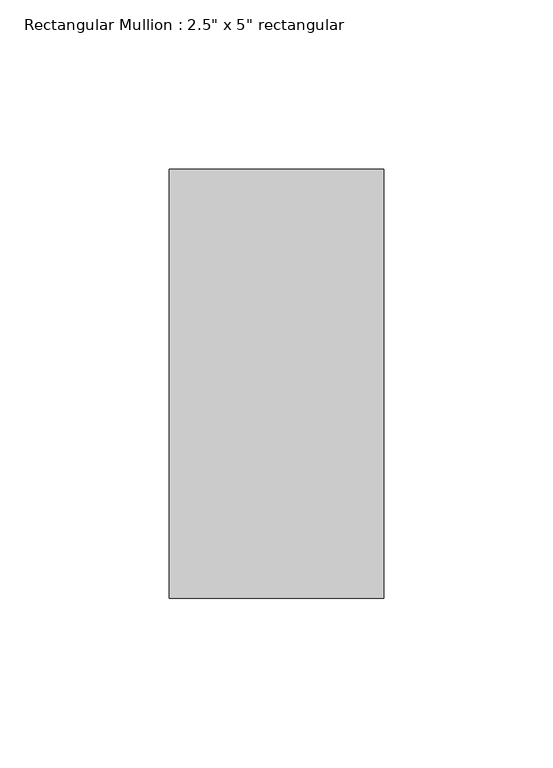
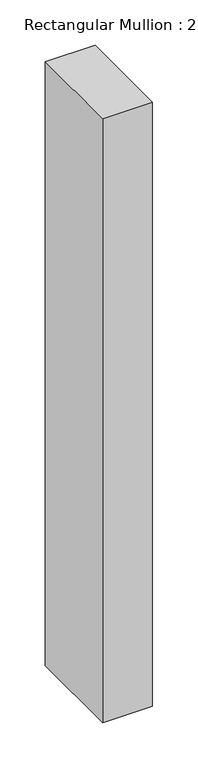
"""IFC4 building model written with IfcOpenShell, lengths in millimetres: member geometry."""

from ifc_helpers import new_model, si_unit, frame, origin, place, context, project, spatial, polyline, outline, extrude, source, transform, mapped, element, save


def member_08dd3726(model_context):
    return source(origin(), model_context, "Body", "SweptSolid", [
        extrude(outline(polyline([(31.75, 63.5), (31.75, -63.5), (-31.75, -63.5), (-31.75, 63.5), (31.75, 63.5)])), frame((0.0, 0.0, -814.5761324), z_axis=(0.0, 0.0, 1.0), x_axis=(1.0, 0.0, 0.0)), (0.0, 0.0, 1.0), 814.5761324),
    ])


if __name__ == "__main__":
    model = new_model("IFC4")
    model_context = context("Model", 3, world=origin())
    ifc_project = project(units=[si_unit("LENGTHUNIT", "METRE", prefix="MILLI")], contexts=[model_context])
    site = spatial("IfcSite", under=ifc_project)
    building = spatial("IfcBuilding", under=site)
    placement = place(None, origin())
    member_shape = member_08dd3726(model_context)
    element("IfcMember", 1, ObjectType="Rectangular Mullion : 2.5\" x 5\" rectangular", at=placement, inside=building, context=model_context, shape_type="MappedRepresentation", body=[
        mapped(member_shape, transform((0.0, 0.0, 0.0), x_axis=(1.0, 0.0, 0.0), y_axis=(0.0, 1.0, 0.0), z_axis=(0.0, 0.0, 1.0))),
    ])
    save(model, "model.ifc")

# Revit data of these elements
# Type "Rectangular Mullion : 2.5\" x 5\" rectangular"
#   built-in parameter 1007304 = 0.416667 (stored number, unit not read)
#   built-in parameter 1007301 = 0.104167 (stored number, unit not read)
#   built-in parameter 1007300 = 0.104167 (stored number, unit not read)
# Element 1 (IfcMember, "Rectangular Mullion : 2.5\" x 5\" rectangular")
#   Materials on its faces: "Aluminum"
# Materials
#   "Aluminum": class "Metal", colour RGB 247 247 247, transparency 0, Description = "Aluminum 6061", Cost = 0
